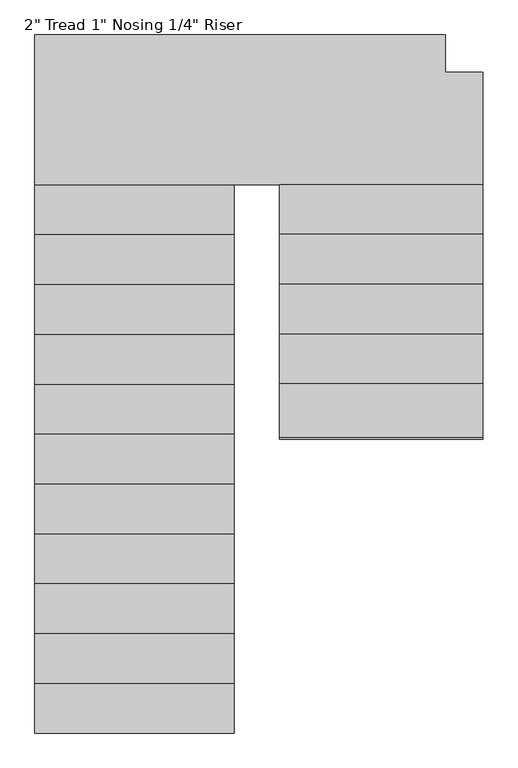
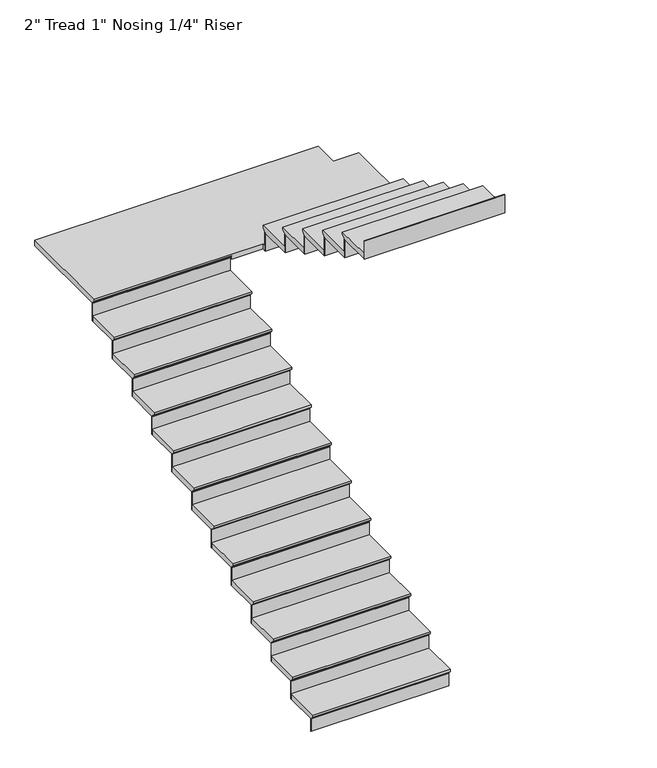
"""IFC4 building model written with IfcOpenShell, lengths in millimetres: stair flight geometry."""

from ifc_helpers import new_model, si_unit, origin, place, context, project, spatial, faceted_brep, source, transform, mapped, element, save


def stair_flight_75ba705f(model_context):
    return source(origin(), model_context, "Body", "Brep", [
        faceted_brep([(-1810.3456086, -4300.9794704, 9599.0833333), (-1810.3456086, -4300.9794704, 9618.1333333), (-3029.5456086, -4300.9794704, 9618.1333333), (-3029.5456086, -4300.9794704, 9599.0833333), (-1810.3456086, -4275.5794704, 9573.6833333), (-3029.5456086, -4275.5794704, 9573.6833333), (-1810.3456086, -3970.7794704, 9618.1333333), (-3029.5456086, -3970.7794704, 9618.1333333), (-3029.5456086, -4275.5794704, 9567.3333333), (-3029.5456086, -3970.7794704, 9567.3333333), (-1810.3456086, -3970.7794704, 9567.3333333), (-1810.3456086, -4275.5794704, 9567.3333333)], [[[0, 1, 2, 3]], [[4, 0, 3, 5]], [[2, 1, 6, 7]], [[8, 9, 10, 11]], [[2, 7, 9, 8, 5, 3]], [[8, 11, 4, 5]], [[6, 1, 0, 4, 11, 10]], [[7, 6, 10, 9]]]),
        faceted_brep([(-1810.3456086, -4275.5794704, 9567.3333333), (-1810.3456086, -4275.5794704, 9448.8), (-1810.3456086, -4269.2294704, 9448.8), (-1810.3456086, -4269.2294704, 9567.3333333), (-3029.5456086, -4275.5794704, 9567.3333333), (-3029.5456086, -4269.2294704, 9567.3333333), (-3029.5456086, -4269.2294704, 9448.8), (-3029.5456086, -4275.5794704, 9448.8)], [[[0, 1, 2, 3]], [[4, 5, 6, 7]], [[1, 0, 4, 7]], [[2, 1, 7, 6]], [[3, 2, 6, 5]], [[0, 3, 5, 4]]]),
        faceted_brep([(-1810.3456086, -3970.7794704, 9736.6666667), (-1810.3456086, -3970.7794704, 9567.3333333), (-1810.3456086, -3964.4294704, 9567.3333333), (-1810.3456086, -3964.4294704, 9736.6666667), (-3029.5456086, -3970.7794704, 9736.6666667), (-3029.5456086, -3964.4294704, 9736.6666667), (-3029.5456086, -3964.4294704, 9567.3333333), (-3029.5456086, -3970.7794704, 9567.3333333)], [[[0, 1, 2, 3]], [[4, 5, 6, 7]], [[1, 0, 4, 7]], [[2, 1, 7, 6]], [[3, 2, 6, 5]], [[0, 3, 5, 4]]]),
        faceted_brep([(-3029.5456086, -3996.1794704, 9787.4666667), (-1810.3456086, -3996.1794704, 9787.4666667), (-1810.3456086, -3665.9794704, 9787.4666667), (-3029.5456086, -3665.9794704, 9787.4666667), (-3029.5456086, -3970.7794704, 9736.6666667), (-3029.5456086, -3665.9794704, 9736.6666667), (-1810.3456086, -3665.9794704, 9736.6666667), (-1810.3456086, -3970.7794704, 9736.6666667), (-3029.5456086, -3970.7794704, 9743.0166667), (-3029.5456086, -3996.1794704, 9768.4166667), (-1810.3456086, -3970.7794704, 9743.0166667), (-1810.3456086, -3996.1794704, 9768.4166667)], [[[0, 1, 2, 3]], [[4, 5, 6, 7]], [[0, 3, 5, 4, 8, 9]], [[4, 7, 10, 8]], [[2, 1, 11, 10, 7, 6]], [[3, 2, 6, 5]], [[11, 1, 0, 9]], [[10, 11, 9, 8]]]),
        faceted_brep([(-1810.3456086, -3665.9794704, 9906.0), (-1810.3456086, -3665.9794704, 9736.6666667), (-1810.3456086, -3659.6294704, 9736.6666667), (-1810.3456086, -3659.6294704, 9906.0), (-3029.5456086, -3665.9794704, 9906.0), (-3029.5456086, -3659.6294704, 9906.0), (-3029.5456086, -3659.6294704, 9736.6666667), (-3029.5456086, -3665.9794704, 9736.6666667)], [[[0, 1, 2, 3]], [[4, 5, 6, 7]], [[1, 0, 4, 7]], [[2, 1, 7, 6]], [[3, 2, 6, 5]], [[0, 3, 5, 4]]]),
        faceted_brep([(-3029.5456086, -3691.3794704, 9956.8), (-1810.3456086, -3691.3794704, 9956.8), (-1810.3456086, -3361.1794704, 9956.8), (-3029.5456086, -3361.1794704, 9956.8), (-3029.5456086, -3665.9794704, 9906.0), (-3029.5456086, -3361.1794704, 9906.0), (-1810.3456086, -3361.1794704, 9906.0), (-1810.3456086, -3665.9794704, 9906.0), (-3029.5456086, -3665.9794704, 9912.35), (-3029.5456086, -3691.3794704, 9937.75), (-1810.3456086, -3665.9794704, 9912.35), (-1810.3456086, -3691.3794704, 9937.75)], [[[0, 1, 2, 3]], [[4, 5, 6, 7]], [[0, 3, 5, 4, 8, 9]], [[4, 7, 10, 8]], [[2, 1, 11, 10, 7, 6]], [[3, 2, 6, 5]], [[11, 1, 0, 9]], [[10, 11, 9, 8]]]),
        faceted_brep([(-1810.3456086, -3361.1794704, 10075.3333333), (-1810.3456086, -3361.1794704, 9906.0), (-1810.3456086, -3354.8294704, 9906.0), (-1810.3456086, -3354.8294704, 10075.3333333), (-3029.5456086, -3361.1794704, 10075.3333333), (-3029.5456086, -3354.8294704, 10075.3333333), (-3029.5456086, -3354.8294704, 9906.0), (-3029.5456086, -3361.1794704, 9906.0)], [[[0, 1, 2, 3]], [[4, 5, 6, 7]], [[1, 0, 4, 7]], [[2, 1, 7, 6]], [[3, 2, 6, 5]], [[0, 3, 5, 4]]]),
        faceted_brep([(-3029.5456086, -3386.5794704, 10126.1333333), (-1810.3456086, -3386.5794704, 10126.1333333), (-1810.3456086, -3056.3794704, 10126.1333333), (-3029.5456086, -3056.3794704, 10126.1333333), (-3029.5456086, -3361.1794704, 10075.3333333), (-3029.5456086, -3056.3794704, 10075.3333333), (-1810.3456086, -3056.3794704, 10075.3333333), (-1810.3456086, -3361.1794704, 10075.3333333), (-3029.5456086, -3361.1794704, 10081.6833333), (-3029.5456086, -3386.5794704, 10107.0833333), (-1810.3456086, -3361.1794704, 10081.6833333), (-1810.3456086, -3386.5794704, 10107.0833333)], [[[0, 1, 2, 3]], [[4, 5, 6, 7]], [[0, 3, 5, 4, 8, 9]], [[4, 7, 10, 8]], [[2, 1, 11, 10, 7, 6]], [[3, 2, 6, 5]], [[11, 1, 0, 9]], [[10, 11, 9, 8]]]),
        faceted_brep([(-1810.3456086, -3056.3794704, 10244.6666667), (-1810.3456086, -3056.3794704, 10075.3333333), (-1810.3456086, -3050.0294704, 10075.3333333), (-1810.3456086, -3050.0294704, 10244.6666667), (-3029.5456086, -3056.3794704, 10244.6666667), (-3029.5456086, -3050.0294704, 10244.6666667), (-3029.5456086, -3050.0294704, 10075.3333333), (-3029.5456086, -3056.3794704, 10075.3333333)], [[[0, 1, 2, 3]], [[4, 5, 6, 7]], [[1, 0, 4, 7]], [[2, 1, 7, 6]], [[3, 2, 6, 5]], [[0, 3, 5, 4]]]),
        faceted_brep([(-3029.5456086, -3081.7794704, 10295.4666667), (-1810.3456086, -3081.7794704, 10295.4666667), (-1810.3456086, -2751.5794704, 10295.4666667), (-3029.5456086, -2751.5794704, 10295.4666667), (-3029.5456086, -3056.3794704, 10244.6666667), (-3029.5456086, -2751.5794704, 10244.6666667), (-1810.3456086, -2751.5794704, 10244.6666667), (-1810.3456086, -3056.3794704, 10244.6666667), (-3029.5456086, -3056.3794704, 10251.0166667), (-3029.5456086, -3081.7794704, 10276.4166667), (-1810.3456086, -3056.3794704, 10251.0166667), (-1810.3456086, -3081.7794704, 10276.4166667)], [[[0, 1, 2, 3]], [[4, 5, 6, 7]], [[0, 3, 5, 4, 8, 9]], [[4, 7, 10, 8]], [[2, 1, 11, 10, 7, 6]], [[3, 2, 6, 5]], [[11, 1, 0, 9]], [[10, 11, 9, 8]]]),
        faceted_brep([(-1810.3456086, -2751.5794704, 10414.0), (-1810.3456086, -2751.5794704, 10244.6666667), (-1810.3456086, -2745.2294704, 10244.6666667), (-1810.3456086, -2745.2294704, 10414.0), (-3029.5456086, -2751.5794704, 10414.0), (-3029.5456086, -2745.2294704, 10414.0), (-3029.5456086, -2745.2294704, 10244.6666667), (-3029.5456086, -2751.5794704, 10244.6666667)], [[[0, 1, 2, 3]], [[4, 5, 6, 7]], [[1, 0, 4, 7]], [[2, 1, 7, 6]], [[3, 2, 6, 5]], [[0, 3, 5, 4]]]),
        faceted_brep([(-3029.5456086, -2776.9794704, 10464.8), (-1810.3456086, -2776.9794704, 10464.8), (-1810.3456086, -2446.7794704, 10464.8), (-3029.5456086, -2446.7794704, 10464.8), (-3029.5456086, -2751.5794704, 10414.0), (-3029.5456086, -2446.7794704, 10414.0), (-1810.3456086, -2446.7794704, 10414.0), (-1810.3456086, -2751.5794704, 10414.0), (-3029.5456086, -2751.5794704, 10420.35), (-3029.5456086, -2776.9794704, 10445.75), (-1810.3456086, -2751.5794704, 10420.35), (-1810.3456086, -2776.9794704, 10445.75)], [[[0, 1, 2, 3]], [[4, 5, 6, 7]], [[0, 3, 5, 4, 8, 9]], [[4, 7, 10, 8]], [[2, 1, 11, 10, 7, 6]], [[3, 2, 6, 5]], [[11, 1, 0, 9]], [[10, 11, 9, 8]]]),
        faceted_brep([(-1810.3456086, -2446.7794704, 10583.3333333), (-1810.3456086, -2446.7794704, 10414.0), (-1810.3456086, -2440.4294704, 10414.0), (-1810.3456086, -2440.4294704, 10583.3333333), (-3029.5456086, -2446.7794704, 10583.3333333), (-3029.5456086, -2440.4294704, 10583.3333333), (-3029.5456086, -2440.4294704, 10414.0), (-3029.5456086, -2446.7794704, 10414.0)], [[[0, 1, 2, 3]], [[4, 5, 6, 7]], [[1, 0, 4, 7]], [[2, 1, 7, 6]], [[3, 2, 6, 5]], [[0, 3, 5, 4]]]),
        faceted_brep([(-3029.5456086, -2472.1794704, 10634.1333333), (-1810.3456086, -2472.1794704, 10634.1333333), (-1810.3456086, -2141.9794704, 10634.1333333), (-3029.5456086, -2141.9794704, 10634.1333333), (-3029.5456086, -2446.7794704, 10583.3333333), (-3029.5456086, -2141.9794704, 10583.3333333), (-1810.3456086, -2141.9794704, 10583.3333333), (-1810.3456086, -2446.7794704, 10583.3333333), (-3029.5456086, -2446.7794704, 10589.6833333), (-3029.5456086, -2472.1794704, 10615.0833333), (-1810.3456086, -2446.7794704, 10589.6833333), (-1810.3456086, -2472.1794704, 10615.0833333)], [[[0, 1, 2, 3]], [[4, 5, 6, 7]], [[0, 3, 5, 4, 8, 9]], [[4, 7, 10, 8]], [[2, 1, 11, 10, 7, 6]], [[3, 2, 6, 5]], [[11, 1, 0, 9]], [[10, 11, 9, 8]]]),
        faceted_brep([(-1810.3456086, -2141.9794704, 10752.6666667), (-1810.3456086, -2141.9794704, 10583.3333333), (-1810.3456086, -2135.6294704, 10583.3333333), (-1810.3456086, -2135.6294704, 10752.6666667), (-3029.5456086, -2141.9794704, 10752.6666667), (-3029.5456086, -2135.6294704, 10752.6666667), (-3029.5456086, -2135.6294704, 10583.3333333), (-3029.5456086, -2141.9794704, 10583.3333333)], [[[0, 1, 2, 3]], [[4, 5, 6, 7]], [[1, 0, 4, 7]], [[2, 1, 7, 6]], [[3, 2, 6, 5]], [[0, 3, 5, 4]]]),
        faceted_brep([(-3029.5456086, -2167.3794704, 10803.4666667), (-1810.3456086, -2167.3794704, 10803.4666667), (-1810.3456086, -1837.1794704, 10803.4666667), (-3029.5456086, -1837.1794704, 10803.4666667), (-3029.5456086, -2141.9794704, 10752.6666667), (-3029.5456086, -1837.1794704, 10752.6666667), (-1810.3456086, -1837.1794704, 10752.6666667), (-1810.3456086, -2141.9794704, 10752.6666667), (-3029.5456086, -2141.9794704, 10759.0166667), (-3029.5456086, -2167.3794704, 10784.4166667), (-1810.3456086, -2141.9794704, 10759.0166667), (-1810.3456086, -2167.3794704, 10784.4166667)], [[[0, 1, 2, 3]], [[4, 5, 6, 7]], [[0, 3, 5, 4, 8, 9]], [[4, 7, 10, 8]], [[2, 1, 11, 10, 7, 6]], [[3, 2, 6, 5]], [[11, 1, 0, 9]], [[10, 11, 9, 8]]]),
        faceted_brep([(-1810.3456086, -1837.1794704, 10922.0), (-1810.3456086, -1837.1794704, 10752.6666667), (-1810.3456086, -1830.8294704, 10752.6666667), (-1810.3456086, -1830.8294704, 10922.0), (-3029.5456086, -1837.1794704, 10922.0), (-3029.5456086, -1830.8294704, 10922.0), (-3029.5456086, -1830.8294704, 10752.6666667), (-3029.5456086, -1837.1794704, 10752.6666667)], [[[0, 1, 2, 3]], [[4, 5, 6, 7]], [[1, 0, 4, 7]], [[2, 1, 7, 6]], [[3, 2, 6, 5]], [[0, 3, 5, 4]]]),
        faceted_brep([(-3029.5456086, -1862.5794704, 10972.8), (-1810.3456086, -1862.5794704, 10972.8), (-1810.3456086, -1532.3794704, 10972.8), (-3029.5456086, -1532.3794704, 10972.8), (-3029.5456086, -1837.1794704, 10922.0), (-3029.5456086, -1532.3794704, 10922.0), (-1810.3456086, -1532.3794704, 10922.0), (-1810.3456086, -1837.1794704, 10922.0), (-3029.5456086, -1837.1794704, 10928.35), (-3029.5456086, -1862.5794704, 10953.75), (-1810.3456086, -1837.1794704, 10928.35), (-1810.3456086, -1862.5794704, 10953.75)], [[[0, 1, 2, 3]], [[4, 5, 6, 7]], [[0, 3, 5, 4, 8, 9]], [[4, 7, 10, 8]], [[2, 1, 11, 10, 7, 6]], [[3, 2, 6, 5]], [[11, 1, 0, 9]], [[10, 11, 9, 8]]]),
        faceted_brep([(-1810.3456086, -1532.3794704, 11091.3333333), (-1810.3456086, -1532.3794704, 10922.0), (-1810.3456086, -1526.0294704, 10922.0), (-1810.3456086, -1526.0294704, 11091.3333333), (-3029.5456086, -1532.3794704, 11091.3333333), (-3029.5456086, -1526.0294704, 11091.3333333), (-3029.5456086, -1526.0294704, 10922.0), (-3029.5456086, -1532.3794704, 10922.0)], [[[0, 1, 2, 3]], [[4, 5, 6, 7]], [[1, 0, 4, 7]], [[2, 1, 7, 6]], [[3, 2, 6, 5]], [[0, 3, 5, 4]]]),
        faceted_brep([(-3029.5456086, -1557.7794704, 11142.1333333), (-1810.3456086, -1557.7794704, 11142.1333333), (-1810.3456086, -1227.5794704, 11142.1333333), (-3029.5456086, -1227.5794704, 11142.1333333), (-3029.5456086, -1532.3794704, 11091.3333333), (-3029.5456086, -1227.5794704, 11091.3333333), (-1810.3456086, -1227.5794704, 11091.3333333), (-1810.3456086, -1532.3794704, 11091.3333333), (-3029.5456086, -1532.3794704, 11097.6833333), (-3029.5456086, -1557.7794704, 11123.0833333), (-1810.3456086, -1532.3794704, 11097.6833333), (-1810.3456086, -1557.7794704, 11123.0833333)], [[[0, 1, 2, 3]], [[4, 5, 6, 7]], [[0, 3, 5, 4, 8, 9]], [[4, 7, 10, 8]], [[2, 1, 11, 10, 7, 6]], [[3, 2, 6, 5]], [[11, 1, 0, 9]], [[10, 11, 9, 8]]]),
        faceted_brep([(-1810.3456086, -1227.5794704, 11260.6666667), (-1810.3456086, -1227.5794704, 11091.3333333), (-1810.3456086, -1221.2294704, 11091.3333333), (-1810.3456086, -1221.2294704, 11260.6666667), (-3029.5456086, -1227.5794704, 11260.6666667), (-3029.5456086, -1221.2294704, 11260.6666667), (-3029.5456086, -1221.2294704, 11091.3333333), (-3029.5456086, -1227.5794704, 11091.3333333)], [[[0, 1, 2, 3]], [[4, 5, 6, 7]], [[1, 0, 4, 7]], [[2, 1, 7, 6]], [[3, 2, 6, 5]], [[0, 3, 5, 4]]]),
        faceted_brep([(-3029.5456086, -1252.9794704, 11311.4666667), (-1810.3456086, -1252.9794704, 11311.4666667), (-1810.3456086, -922.7794704, 11311.4666667), (-3029.5456086, -922.7794704, 11311.4666667), (-3029.5456086, -1227.5794704, 11260.6666667), (-3029.5456086, -922.7794704, 11260.6666667), (-1810.3456086, -922.7794704, 11260.6666667), (-1810.3456086, -1227.5794704, 11260.6666667), (-3029.5456086, -1227.5794704, 11267.0166667), (-3029.5456086, -1252.9794704, 11292.4166667), (-1810.3456086, -1227.5794704, 11267.0166667), (-1810.3456086, -1252.9794704, 11292.4166667)], [[[0, 1, 2, 3]], [[4, 5, 6, 7]], [[0, 3, 5, 4, 8, 9]], [[4, 7, 10, 8]], [[2, 1, 11, 10, 7, 6]], [[3, 2, 6, 5]], [[11, 1, 0, 9]], [[10, 11, 9, 8]]]),
        faceted_brep([(-1810.3456086, -922.7794704, 11430.0), (-1810.3456086, -922.7794704, 11260.6666667), (-1810.3456086, -916.4294704, 11260.6666667), (-1810.3456086, -916.4294704, 11430.0), (-3029.5456086, -922.7794704, 11430.0), (-3029.5456086, -916.4294704, 11430.0), (-3029.5456086, -916.4294704, 11260.6666667), (-3029.5456086, -922.7794704, 11260.6666667)], [[[0, 1, 2, 3]], [[4, 5, 6, 7]], [[1, 0, 4, 7]], [[2, 1, 7, 6]], [[3, 2, 6, 5]], [[0, 3, 5, 4]]]),
        faceted_brep([(-289.8083398, -973.5794704, 11480.8), (-289.8083398, -262.3794704, 11480.8), (-518.4083398, -262.3794704, 11480.8), (-518.4083398, -33.7794704, 11480.8), (-3029.5456086, -33.7794704, 11480.8), (-3029.5456086, -948.1794704, 11480.8), (-1534.4083398, -948.1794704, 11480.8), (-1534.4083398, -973.5794704, 11480.8), (-289.8083398, -262.3794704, 11430.0), (-289.8083398, -973.5794704, 11430.0), (-1534.4083398, -973.5794704, 11430.0), (-1534.4083398, -948.1794704, 11430.0), (-1810.3456086, -948.1794704, 11430.0), (-1810.3456086, -922.7794704, 11430.0), (-3029.5456086, -922.7794704, 11430.0), (-3029.5456086, -33.7794704, 11430.0), (-518.4083398, -33.7794704, 11430.0), (-518.4083398, -262.3794704, 11430.0), (-3029.5456086, -922.7794704, 11436.35), (-3029.5456086, -948.1794704, 11461.75), (-1810.3456086, -922.7794704, 11436.35), (-1810.3456086, -948.1794704, 11461.75)], [[[0, 1, 2, 3, 4, 5, 6, 7]], [[8, 9, 10, 11, 12, 13, 14, 15, 16, 17]], [[1, 0, 9, 8]], [[2, 1, 8, 17]], [[3, 2, 17, 16]], [[4, 3, 16, 15]], [[5, 4, 15, 14, 18, 19]], [[14, 13, 20, 18]], [[13, 12, 21, 20]], [[6, 5, 19, 21, 12, 11]], [[7, 6, 11, 10]], [[0, 7, 10, 9]], [[19, 18, 20, 21]]]),
        faceted_brep([(-1534.4083398, -973.5794704, 11599.3333333), (-1534.4083398, -973.5794704, 11430.0), (-1534.4083398, -979.9294704, 11430.0), (-1534.4083398, -979.9294704, 11599.3333333), (-289.8083398, -973.5794704, 11599.3333333), (-289.8083398, -979.9294704, 11599.3333333), (-289.8083398, -979.9294704, 11430.0), (-289.8083398, -973.5794704, 11430.0)], [[[0, 1, 2, 3]], [[4, 5, 6, 7]], [[1, 0, 4, 7]], [[2, 1, 7, 6]], [[3, 2, 6, 5]], [[0, 3, 5, 4]]]),
        faceted_brep([(-289.8083398, -948.1794704, 11650.1333333), (-1534.4083398, -948.1794704, 11650.1333333), (-1534.4083398, -1278.3794704, 11650.1333333), (-289.8083398, -1278.3794704, 11650.1333333), (-289.8083398, -973.5794704, 11599.3333333), (-289.8083398, -1278.3794704, 11599.3333333), (-1534.4083398, -1278.3794704, 11599.3333333), (-1534.4083398, -973.5794704, 11599.3333333), (-289.8083398, -973.5794704, 11605.6833333), (-289.8083398, -948.1794704, 11631.0833333), (-1534.4083398, -973.5794704, 11605.6833333), (-1534.4083398, -948.1794704, 11631.0833333)], [[[0, 1, 2, 3]], [[4, 5, 6, 7]], [[0, 3, 5, 4, 8, 9]], [[4, 7, 10, 8]], [[2, 1, 11, 10, 7, 6]], [[3, 2, 6, 5]], [[11, 1, 0, 9]], [[10, 11, 9, 8]]]),
        faceted_brep([(-1534.4083398, -1278.3794704, 11768.6666667), (-1534.4083398, -1278.3794704, 11599.3333333), (-1534.4083398, -1284.7294704, 11599.3333333), (-1534.4083398, -1284.7294704, 11768.6666667), (-289.8083398, -1278.3794704, 11768.6666667), (-289.8083398, -1284.7294704, 11768.6666667), (-289.8083398, -1284.7294704, 11599.3333333), (-289.8083398, -1278.3794704, 11599.3333333)], [[[0, 1, 2, 3]], [[4, 5, 6, 7]], [[1, 0, 4, 7]], [[2, 1, 7, 6]], [[3, 2, 6, 5]], [[0, 3, 5, 4]]]),
        faceted_brep([(-289.8083398, -1252.9794704, 11819.4666667), (-1534.4083398, -1252.9794704, 11819.4666667), (-1534.4083398, -1583.1794704, 11819.4666667), (-289.8083398, -1583.1794704, 11819.4666667), (-289.8083398, -1278.3794704, 11768.6666667), (-289.8083398, -1583.1794704, 11768.6666667), (-1534.4083398, -1583.1794704, 11768.6666667), (-1534.4083398, -1278.3794704, 11768.6666667), (-289.8083398, -1278.3794704, 11775.0166667), (-289.8083398, -1252.9794704, 11800.4166667), (-1534.4083398, -1278.3794704, 11775.0166667), (-1534.4083398, -1252.9794704, 11800.4166667)], [[[0, 1, 2, 3]], [[4, 5, 6, 7]], [[0, 3, 5, 4, 8, 9]], [[4, 7, 10, 8]], [[2, 1, 11, 10, 7, 6]], [[3, 2, 6, 5]], [[11, 1, 0, 9]], [[10, 11, 9, 8]]]),
        faceted_brep([(-1534.4083398, -1583.1794704, 11938.0), (-1534.4083398, -1583.1794704, 11768.6666667), (-1534.4083398, -1589.5294704, 11768.6666667), (-1534.4083398, -1589.5294704, 11938.0), (-289.8083398, -1583.1794704, 11938.0), (-289.8083398, -1589.5294704, 11938.0), (-289.8083398, -1589.5294704, 11768.6666667), (-289.8083398, -1583.1794704, 11768.6666667)], [[[0, 1, 2, 3]], [[4, 5, 6, 7]], [[1, 0, 4, 7]], [[2, 1, 7, 6]], [[3, 2, 6, 5]], [[0, 3, 5, 4]]]),
        faceted_brep([(-289.8083398, -1557.7794704, 11988.8), (-1534.4083398, -1557.7794704, 11988.8), (-1534.4083398, -1887.9794704, 11988.8), (-289.8083398, -1887.9794704, 11988.8), (-289.8083398, -1583.1794704, 11938.0), (-289.8083398, -1887.9794704, 11938.0), (-1534.4083398, -1887.9794704, 11938.0), (-1534.4083398, -1583.1794704, 11938.0), (-289.8083398, -1583.1794704, 11944.35), (-289.8083398, -1557.7794704, 11969.75), (-1534.4083398, -1583.1794704, 11944.35), (-1534.4083398, -1557.7794704, 11969.75)], [[[0, 1, 2, 3]], [[4, 5, 6, 7]], [[0, 3, 5, 4, 8, 9]], [[4, 7, 10, 8]], [[2, 1, 11, 10, 7, 6]], [[3, 2, 6, 5]], [[11, 1, 0, 9]], [[10, 11, 9, 8]]]),
        faceted_brep([(-1534.4083398, -1887.9794704, 12107.3333333), (-1534.4083398, -1887.9794704, 11938.0), (-1534.4083398, -1894.3294704, 11938.0), (-1534.4083398, -1894.3294704, 12107.3333333), (-289.8083398, -1887.9794704, 12107.3333333), (-289.8083398, -1894.3294704, 12107.3333333), (-289.8083398, -1894.3294704, 11938.0), (-289.8083398, -1887.9794704, 11938.0)], [[[0, 1, 2, 3]], [[4, 5, 6, 7]], [[1, 0, 4, 7]], [[2, 1, 7, 6]], [[3, 2, 6, 5]], [[0, 3, 5, 4]]]),
        faceted_brep([(-289.8083398, -1862.5794704, 12158.1333333), (-1534.4083398, -1862.5794704, 12158.1333333), (-1534.4083398, -2192.7794704, 12158.1333333), (-289.8083398, -2192.7794704, 12158.1333333), (-289.8083398, -1887.9794704, 12107.3333333), (-289.8083398, -2192.7794704, 12107.3333333), (-1534.4083398, -2192.7794704, 12107.3333333), (-1534.4083398, -1887.9794704, 12107.3333333), (-289.8083398, -1887.9794704, 12113.6833333), (-289.8083398, -1862.5794704, 12139.0833333), (-1534.4083398, -1887.9794704, 12113.6833333), (-1534.4083398, -1862.5794704, 12139.0833333)], [[[0, 1, 2, 3]], [[4, 5, 6, 7]], [[0, 3, 5, 4, 8, 9]], [[4, 7, 10, 8]], [[2, 1, 11, 10, 7, 6]], [[3, 2, 6, 5]], [[11, 1, 0, 9]], [[10, 11, 9, 8]]]),
        faceted_brep([(-1534.4083398, -2192.7794704, 12276.6666667), (-1534.4083398, -2192.7794704, 12107.3333333), (-1534.4083398, -2199.1294704, 12107.3333333), (-1534.4083398, -2199.1294704, 12276.6666667), (-289.8083398, -2192.7794704, 12276.6666667), (-289.8083398, -2199.1294704, 12276.6666667), (-289.8083398, -2199.1294704, 12107.3333333), (-289.8083398, -2192.7794704, 12107.3333333)], [[[0, 1, 2, 3]], [[4, 5, 6, 7]], [[1, 0, 4, 7]], [[2, 1, 7, 6]], [[3, 2, 6, 5]], [[0, 3, 5, 4]]]),
        faceted_brep([(-1534.4083398, -2497.5794704, 12446.0), (-1534.4083398, -2497.5794704, 12276.6666667), (-1534.4083398, -2503.9294704, 12276.6666667), (-1534.4083398, -2503.9294704, 12446.0), (-289.8083398, -2497.5794704, 12446.0), (-289.8083398, -2503.9294704, 12446.0), (-289.8083398, -2503.9294704, 12276.6666667), (-289.8083398, -2497.5794704, 12276.6666667)], [[[0, 1, 2, 3]], [[4, 5, 6, 7]], [[1, 0, 4, 7]], [[2, 1, 7, 6]], [[3, 2, 6, 5]], [[0, 3, 5, 4]]]),
        faceted_brep([(-289.8083398, -2167.3794704, 12327.4666667), (-1534.4083398, -2167.3794704, 12327.4666667), (-1534.4083398, -2497.5794704, 12327.4666667), (-289.8083398, -2497.5794704, 12327.4666667), (-289.8083398, -2192.7794704, 12276.6666667), (-289.8083398, -2497.5794704, 12276.6666667), (-1534.4083398, -2497.5794704, 12276.6666667), (-1534.4083398, -2192.7794704, 12276.6666667), (-289.8083398, -2192.7794704, 12283.0166667), (-289.8083398, -2167.3794704, 12308.4166667), (-1534.4083398, -2192.7794704, 12283.0166667), (-1534.4083398, -2167.3794704, 12308.4166667)], [[[0, 1, 2, 3]], [[4, 5, 6, 7]], [[0, 3, 5, 4, 8, 9]], [[4, 7, 10, 8]], [[2, 1, 11, 10, 7, 6]], [[3, 2, 6, 5]], [[11, 1, 0, 9]], [[10, 11, 9, 8]]]),
    ])


if __name__ == "__main__":
    model = new_model("IFC4")
    model_context = context("Model", 3, world=origin())
    ifc_project = project(units=[si_unit("LENGTHUNIT", "METRE", prefix="MILLI")], contexts=[model_context])
    site = spatial("IfcSite", under=ifc_project)
    building = spatial("IfcBuilding", under=site)
    placement = place(None, origin())
    stair_flight_shape = stair_flight_75ba705f(model_context)
    element("IfcStairFlight", 1, ObjectType="2\" Tread 1\" Nosing 1/4\" Riser", at=placement, inside=building, context=model_context, shape_type="MappedRepresentation", body=[
        mapped(stair_flight_shape, transform((0.0, 0.0, 0.0), x_axis=(1.0, 0.0, 0.0), y_axis=(0.0, 1.0, 0.0), z_axis=(0.0, 0.0, 1.0))),
    ])
    save(model, "model.ifc")
